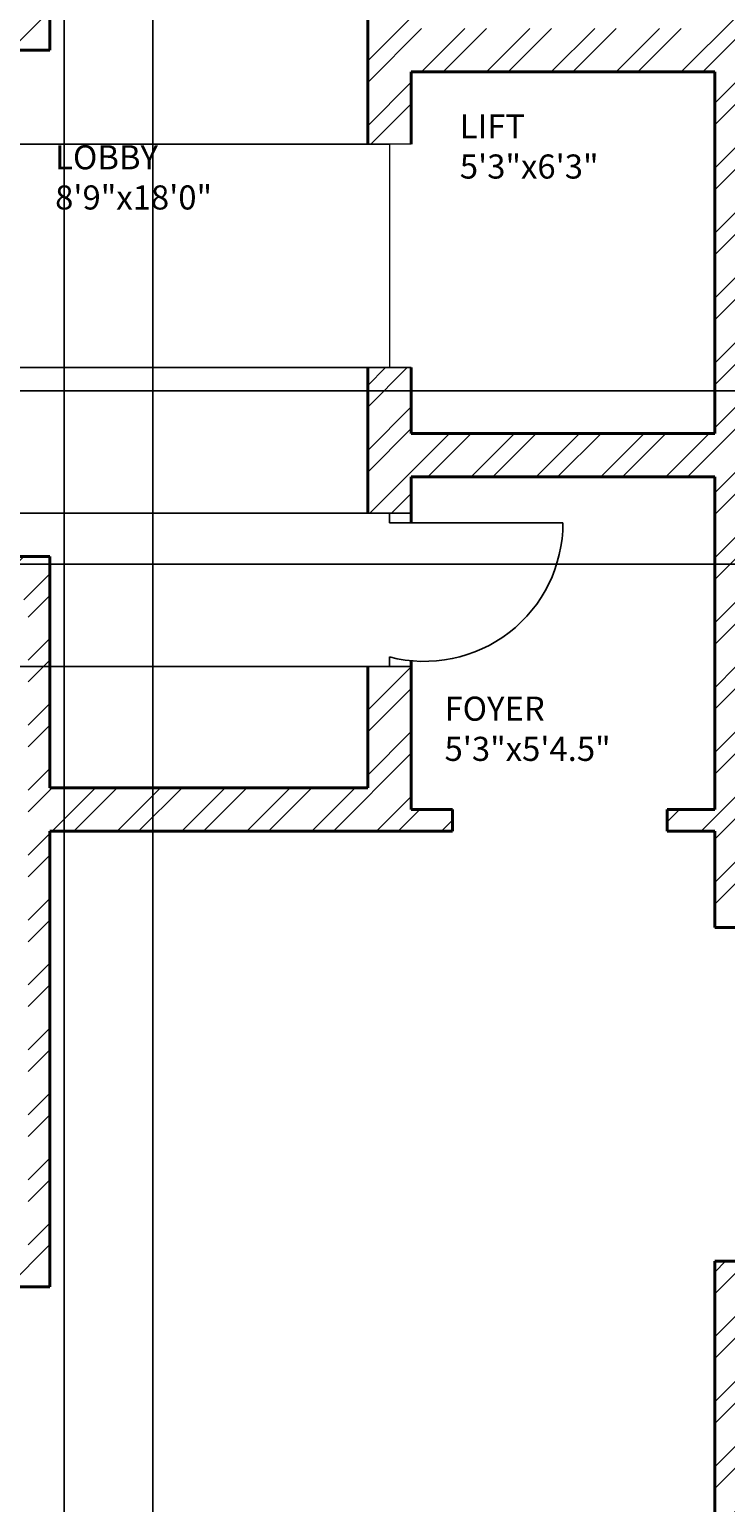
# Model space of a CAD drawing. Units: inches. Extents: x 1601 to 2297, y 1496 to 2631.
# Tile 15 of 57: x 1889 to 2033, y 1835 to 2141. Entities that reach past the tile are written whole.
import ezdxf

# ---------------------------------------------------------------- set-up
doc = ezdxf.new("R2010")
doc.units = ezdxf.units.IN
for name, color, linetype, lineweight in [('A-ANNO-DIMS', 2, 'Continuous', 18), ('A-AREA-IDEN', 7, 'Continuous', 18), ('A-DOOR', 21, 'Continuous', 25), ('A-FLOR-EVTR', 4, 'Continuous', 20), ('A-WALL', 7, 'Continuous', 40), ('A-WALL-PATT', 215, 'Continuous', 13)]:
    doc.layers.add(name, color=color, linetype=linetype, lineweight=lineweight)
doc.styles.get("Standard").update_dxf_attribs({"font": 'arial.ttf'})
doc.dimstyles.get("Standard").update_dxf_attribs({"dimtxt": 0.18, "dimasz": 0.18, "dimexe": 0.18, "dimexo": 0.0625, "dimgap": 0.09, "dimtad": 0, "dimtih": 1, "dimtoh": 1, "dimdec": 4, "dimzin": 0, "dimdsep": 46, "dimtxsty": 'Standard', "dimcen": 0.09, "dimadec": 0, "dimazin": 0, "dimtfac": 1, "dimtdec": 4, "dimtofl": 0, "dimtmove": 0, "dimatfit": 3, "dimfxl": 1, "dimtolj": 1, "dimtzin": 0, "dimarcsym": 0})

# ---------------------------------------------------------------- blocks, each defined once
blk = doc.blocks.new('*D42')
at = {"layer": 'A-ANNO-DIMS', "color": 0, "lineweight": -2, "transparency": 16777216}
for p, q in [((2177.97, 2065.7), (1637.31, 2065.7)), ((1637.49, 2065.52), (1637.49, 2047.88)), ((1637.49, 2029.88), (1637.49, 2047.51)), ((2177.97, 2029.7), (1637.31, 2029.7))]:
    blk.add_line(p, q, dxfattribs=at)
at = {"layer": 'A-ANNO-DIMS', "color": 0, "transparency": 16777216}
for points in [[(1637.46, 2065.52), (1637.52, 2065.52), (1637.49, 2065.7)], [(1637.46, 2029.88), (1637.52, 2029.88), (1637.49, 2029.7)]]:
    blk.add_solid(points, dxfattribs=at)
at = {"layer": 'Defpoints', "color": 0, "transparency": 16777216}
for p in [(1637.49, 2065.7), (2178.04, 2065.7), (2178.04, 2029.7)]:
    blk.add_point(p, dxfattribs=at)
at = {"layer": 'A-ANNO-DIMS', "color": 0, "transparency": 16777216, "insert": (1637.49, 2047.7), "char_height": 0.18, "attachment_point": 5}
blk.add_mtext('\\A1;36', dxfattribs=at)
blk = doc.blocks.new('*D44')
at = {"layer": 'A-ANNO-DIMS', "color": 0, "lineweight": -2, "transparency": 16777216}
for p, q in [((1958.97, 2116.84), (1637.31, 2116.84)), ((1637.49, 2116.66), (1637.49, 2093.85)), ((1637.49, 2070.67), (1637.49, 2093.48)), ((1958.97, 2070.49), (1637.31, 2070.49))]:
    blk.add_line(p, q, dxfattribs=at)
at = {"layer": 'A-ANNO-DIMS', "color": 0, "transparency": 16777216}
for points in [[(1637.46, 2116.66), (1637.52, 2116.66), (1637.49, 2116.84)], [(1637.46, 2070.67), (1637.52, 2070.67), (1637.49, 2070.49)]]:
    blk.add_solid(points, dxfattribs=at)
at = {"layer": 'Defpoints', "color": 0, "transparency": 16777216}
for p in [(1637.49, 2116.84), (1959.04, 2116.84), (1959.04, 2070.49)]:
    blk.add_point(p, dxfattribs=at)
at = {"layer": 'A-ANNO-DIMS', "color": 0, "transparency": 16777216, "insert": (1637.49, 2093.67), "char_height": 0.18, "attachment_point": 5}
blk.add_mtext('\\A1;46.34', dxfattribs=at)
blk = doc.blocks.new('*D45')
at = {"layer": 'A-ANNO-DIMS', "color": 0, "lineweight": -2, "transparency": 16777216}
for p, q in [((1958.97, 2040.3), (1637.31, 2040.3)), ((1637.49, 2040.12), (1637.49, 2024.57)), ((1637.49, 2008.66), (1637.49, 2024.21)), ((1958.97, 2008.48), (1637.31, 2008.48))]:
    blk.add_line(p, q, dxfattribs=at)
at = {"layer": 'A-ANNO-DIMS', "color": 0, "transparency": 16777216}
for points in [[(1637.46, 2040.12), (1637.52, 2040.12), (1637.49, 2040.3)], [(1637.46, 2008.66), (1637.52, 2008.66), (1637.49, 2008.48)]]:
    blk.add_solid(points, dxfattribs=at)
at = {"layer": 'Defpoints', "color": 0, "transparency": 16777216}
for p in [(1637.49, 2040.3), (1959.04, 2040.3), (1959.04, 2008.48)]:
    blk.add_point(p, dxfattribs=at)
at = {"layer": 'A-ANNO-DIMS', "color": 0, "transparency": 16777216, "insert": (1637.49, 2024.39), "char_height": 0.18, "attachment_point": 5}
blk.add_mtext('\\A1;31.83', dxfattribs=at)
blk = doc.blocks.new('*D50')
at = {"layer": 'A-ANNO-DIMS', "color": 0, "lineweight": -2, "transparency": 16777216}
for p, q in [((1895.99, 2374.33), (1895.99, 1513.75)), ((1914.39, 2374.33), (1914.39, 1513.75)), ((1896.17, 1513.93), (1904.87, 1513.93)), ((1914.21, 1513.93), (1905.5, 1513.93))]:
    blk.add_line(p, q, dxfattribs=at)
at = {"layer": 'A-ANNO-DIMS', "color": 0, "transparency": 16777216}
for points in [[(1896.17, 1513.96), (1896.17, 1513.9), (1895.99, 1513.93)], [(1914.21, 1513.96), (1914.21, 1513.9), (1914.39, 1513.93)]]:
    blk.add_solid(points, dxfattribs=at)
at = {"layer": 'Defpoints', "color": 0, "transparency": 16777216}
for p in [(1895.99, 2374.4), (1914.39, 2374.4), (1914.39, 1513.93)]:
    blk.add_point(p, dxfattribs=at)
at = {"layer": 'A-ANNO-DIMS', "color": 0, "transparency": 16777216, "insert": (1905.19, 1513.93), "char_height": 0.18, "attachment_point": 5}
blk.add_mtext('\\A1;18.4', dxfattribs=at)

msp = doc.modelspace()

# ---------------------------------------------------------------- hatches: boundary and pattern name
at = {"layer": 'A-WALL-PATT'}
h = msp.add_hatch(dxfattribs=at)
h.set_pattern_fill('ANSI32', color=256)
h.paths.add_polyline_path([(1842.0336, 2528.0767), (1842.0336, 2532.3254), (1686.0373, 2532.3254), (1686.0373, 2492.9493), (1695.0373, 2492.9493), (1695.0373, 2523.3254), (1827.0373, 2523.3254), (1827.0373, 2416.8254), (1834.6225, 2416.8254), (1834.6225, 2419.0754), (1834.6225, 2421.3254), (1831.5373, 2421.3254), (1831.5373, 2523.3254), (1842.0336, 2523.3254)])
h.paths.add_polyline_path([(1695.0373, 2432.9493), (1686.0373, 2432.9493), (1686.0373, 2325.989), (1695.0373, 2325.989), (1695.0373, 2347.8254), (1827.0373, 2347.8254), (1827.0373, 2287.8254), (1823.2991, 2287.8254), (1823.2991, 2283.3254), (1847.9422, 2283.3254), (1847.9422, 2285.5754), (1847.9422, 2287.8254), (1831.5373, 2287.8254), (1831.5373, 2347.8254), (1846.9946, 2347.8254), (1846.9946, 2350.0754), (1846.9946, 2352.3254), (1695.0373, 2352.3254)])
h.paths.add_polyline_path([(1807.1169, 1573.5395), (2055.0405, 1573.5395), (2055.0405, 1610.6322), (1807.1169, 1610.6322)], flags=9)
h.paths.add_polyline_path([(1841.1631, 1712.7967), (1870.3957, 1712.7967), (1870.3957, 1731.454), (1841.1631, 1731.454)], flags=9)
h.paths.add_polyline_path([(2144.3862, 1772.185), (2191.0233, 1772.185), (2191.0233, 1790.8423), (2144.3862, 1790.8423)], flags=9)
h.paths.add_polyline_path([(2143.0128, 1827.3312), (2177.9958, 1827.3312), (2177.9958, 1845.9886), (2143.0128, 1845.9886)], flags=9)
h.paths.add_polyline_path([(2041.2439, 1833.5691), (2070.8516, 1833.5691), (2070.8516, 1852.2264), (2041.2439, 1852.2264)], flags=9)
h.paths.add_polyline_path([(2097.2791, 1947.0598), (2134.2061, 1947.0598), (2134.2061, 1965.7171), (2097.2791, 1965.7171)], flags=9)
h.paths.add_polyline_path([(2214.995, 1904.3124), (2214.995, 1942.2899), (2196.3376, 1942.2899), (2196.3376, 1904.3124)], flags=9)
h.paths.add_polyline_path([(2186.6284, 2043.8031), (2219.7935, 2043.8031), (2219.7935, 2062.4605), (2186.6284, 2062.4605)], flags=9)
h.paths.add_polyline_path([(2064.0877, 2031.616), (2097.4949, 2031.616), (2097.4949, 2050.2734), (2064.0877, 2050.2734)], flags=9)
h.paths.add_polyline_path([(1973.1349, 1986.0688), (2008.4009, 1986.0688), (2008.4009, 2004.7261), (1973.1349, 2004.7261)], flags=9)
h.paths.add_polyline_path([(1976.3676, 2106.9635), (2005.7469, 2106.9635), (2005.7469, 2125.6209), (1976.3676, 2125.6209)], flags=9)
h.paths.add_polyline_path([(1991.7852, 2180.4863), (2027.0513, 2180.4863), (2027.0513, 2199.1437), (1991.7852, 2199.1437)], flags=9)
h.paths.add_polyline_path([(2106.1801, 2187.9359), (2152.2101, 2187.9359), (2152.2101, 2206.5932), (2106.1801, 2206.5932)], flags=9)
h.paths.add_polyline_path([(2148.6686, 2262.2542), (2182.318, 2262.2542), (2182.318, 2280.9115), (2148.6686, 2280.9115)], flags=9)
h.paths.add_polyline_path([(2041.6327, 2252.8147), (2071.2405, 2252.8147), (2071.2405, 2271.4721), (2041.6327, 2271.4721)], flags=9)
h.paths.add_polyline_path([(2063.9734, 2375.4265), (2100.9004, 2375.4265), (2100.9004, 2394.0839), (2063.9734, 2394.0839)], flags=9)
h.paths.add_polyline_path([(2216.4955, 2330.9748), (2216.4955, 2370.2654), (2197.8381, 2370.2654), (2197.8381, 2330.9748)], flags=9)
h.paths.add_polyline_path([(2179.1416, 2485.8687), (2212.3067, 2485.8687), (2212.3067, 2504.5261), (2179.1416, 2504.5261)], flags=9)
h.paths.add_polyline_path([(2078.7442, 2471.1516), (2112.1514, 2471.1516), (2112.1514, 2489.809), (2078.7442, 2489.809)], flags=9)
h.paths.add_polyline_path([(1915.9631, 2329.4668), (1952.8902, 2329.4668), (1952.8902, 2348.1241), (1915.9631, 2348.1241)], flags=9)
h.paths.add_polyline_path([(1904.3189, 2499.6709), (1940.4512, 2499.6709), (1940.4512, 2518.3282), (1904.3189, 2518.3282)], flags=9)
h.paths.add_polyline_path([(1892.3665, 2100.4595), (1925.6374, 2100.4595), (1925.6374, 2119.1169), (1892.3665, 2119.1169)], flags=9)
h.paths.add_polyline_path([(1909.2984, 1805.9631), (1946.2254, 1805.9631), (1946.2254, 1824.6205), (1909.2984, 1824.6205)], flags=9)
h.paths.add_polyline_path([(1934.6056, 1658.616), (1970.738, 1658.616), (1970.738, 1677.2733), (1934.6056, 1677.2733)], flags=9)
h.paths.add_polyline_path([(1711.2052, 1789.8902), (1750.0456, 1789.8902), (1750.0456, 1808.5476), (1711.2052, 1808.5476)], flags=9)
h.paths.add_polyline_path([(1742.7874, 1854.6743), (1771.9449, 1854.6743), (1771.9449, 1873.3317), (1742.7874, 1873.3317)], flags=9)
h.paths.add_polyline_path([(1807.3592, 1997.7912), (1850.1116, 1997.7912), (1850.1116, 2016.4486), (1807.3592, 2016.4486)], flags=9)
h.paths.add_polyline_path([(1717.4579, 2237.7844), (1760.2103, 2237.7844), (1760.2103, 2256.4417), (1717.4579, 2256.4417)], flags=9)
h.paths.add_polyline_path([(1780.9285, 2324.0623), (1810.086, 2324.0623), (1810.086, 2342.7197), (1780.9285, 2342.7197)], flags=25)
h.paths.add_polyline_path([(1837.696, 2449.2024), (1866.9286, 2449.2024), (1866.9286, 2467.8598), (1837.696, 2467.8598)], flags=9)
h.paths.add_polyline_path([(1712.7752, 2484.9404), (1751.6156, 2484.9404), (1751.6156, 2503.5977), (1712.7752, 2503.5977)], flags=25)
h = msp.add_hatch(dxfattribs=at)
h.set_pattern_fill('ANSI32', color=256)
h.paths.add_polyline_path([(1973.9371, 2211.3254), (1893.0373, 2211.3254), (1893.0373, 2287.8254), (1884.6167, 2287.8254), (1884.6167, 2285.5754), (1884.6167, 2283.3254), (1888.5373, 2283.3254), (1888.5373, 2145.3254), (1695.0373, 2145.3254), (1695.0373, 2173.8724), (1690.5373, 2173.8724), (1686.0373, 2173.8724), (1686.0373, 2136.3254), (1722.5687, 2136.3254), (1722.5687, 2117.4352), (1731.5687, 2117.4352), (1731.5687, 2136.3254), (1893.0373, 2136.3254), (1893.0373, 2202.3254), (1959.0373, 2202.3254), (1959.0373, 2182.1303), (1968.0373, 2182.1303), (1968.0373, 2202.3254), (1973.9371, 2202.3254)])
h.paths.add_polyline_path([(2094.0373, 2274.6364), (2096.4294, 2274.6364), (2096.4294, 2276.8864), (2096.4294, 2279.1364), (2094.0373, 2279.1364), (2094.0373, 2290.8254), (2094.0373, 2295.3254), (2089.5373, 2295.3254), (2089.5373, 2230.8254), (2035.5373, 2230.8254), (2035.5373, 2299.8254), (2031.0373, 2299.8254), (2031.0373, 2211.3254), (2023.0065, 2211.3254), (2023.0065, 2202.3254), (2031.0373, 2202.3254), (2031.0373, 2140.8254), (1968.0373, 2140.8254), (1968.0373, 2145.9106), (1963.5373, 2145.9106), (1959.0373, 2145.9106), (1959.0373, 2116.839), (1963.5373, 2116.839), (1968.0373, 2116.839), (1968.0373, 2131.8254), (2031.0373, 2131.8254), (2031.0373, 2094.3254), (2031.0373, 2085.3254), (2031.0373, 2056.8254), (1968.0373, 2056.8254), (1968.0373, 2070.4947), (1963.5373, 2070.4947), (1959.0373, 2070.4947), (1959.0373, 2040.3029), (1968.0373, 2040.3029), (1968.0373, 2047.8254), (2031.0373, 2047.8254), (2031.0373, 1983.3254), (2031.0373, 1978.8254), (2021.1979, 1978.8254), (2021.1979, 1974.3254), (2031.0373, 1974.3254), (2031.0373, 1954.3528), (2035.5373, 1954.3528), (2035.5373, 1974.3254), (2035.5373, 1981.8254), (2055.5513, 1981.8254), (2055.5513, 1986.3254), (2035.5373, 1986.3254), (2035.5373, 2047.8254), (2040.0373, 2047.8254), (2040.0373, 2085.3254), (2040.0373, 2094.3254), (2040.0373, 2140.8254), (2035.5373, 2140.8254), (2035.5373, 2226.3254), (2089.5373, 2226.3254), (2094.0373, 2226.3254)])
h.paths.add_polyline_path([(2226.0373, 2230.8254), (2134.5373, 2230.8254), (2134.5373, 2233.5437), (2130.0373, 2233.5437), (2130.0373, 2226.3254), (2134.5373, 2226.3254), (2226.0373, 2226.3254)])
h.paths.add_polyline_path([(1807.1169, 1573.5395), (2055.0405, 1573.5395), (2055.0405, 1610.6322), (1807.1169, 1610.6322)], flags=9)
h.paths.add_polyline_path([(1841.1631, 1712.7967), (1870.3957, 1712.7967), (1870.3957, 1731.454), (1841.1631, 1731.454)], flags=9)
h.paths.add_polyline_path([(2144.3862, 1772.185), (2191.0233, 1772.185), (2191.0233, 1790.8423), (2144.3862, 1790.8423)], flags=9)
h.paths.add_polyline_path([(2143.0128, 1827.3312), (2177.9958, 1827.3312), (2177.9958, 1845.9886), (2143.0128, 1845.9886)], flags=9)
h.paths.add_polyline_path([(2041.2439, 1833.5691), (2070.8516, 1833.5691), (2070.8516, 1852.2264), (2041.2439, 1852.2264)], flags=9)
h.paths.add_polyline_path([(2097.2791, 1947.0598), (2134.2061, 1947.0598), (2134.2061, 1965.7171), (2097.2791, 1965.7171)], flags=9)
h.paths.add_polyline_path([(2214.995, 1904.3124), (2214.995, 1942.2899), (2196.3376, 1942.2899), (2196.3376, 1904.3124)], flags=9)
h.paths.add_polyline_path([(2186.6284, 2043.8031), (2219.7935, 2043.8031), (2219.7935, 2062.4605), (2186.6284, 2062.4605)], flags=9)
h.paths.add_polyline_path([(2064.0877, 2031.616), (2097.4949, 2031.616), (2097.4949, 2050.2734), (2064.0877, 2050.2734)], flags=9)
h.paths.add_polyline_path([(1973.1349, 1986.0688), (2008.4009, 1986.0688), (2008.4009, 2004.7261), (1973.1349, 2004.7261)], flags=25)
h.paths.add_polyline_path([(1976.3676, 2106.9635), (2005.7469, 2106.9635), (2005.7469, 2125.6209), (1976.3676, 2125.6209)], flags=25)
h.paths.add_polyline_path([(1991.7852, 2180.4863), (2027.0513, 2180.4863), (2027.0513, 2199.1437), (1991.7852, 2199.1437)], flags=25)
h.paths.add_polyline_path([(2106.1801, 2187.9359), (2152.2101, 2187.9359), (2152.2101, 2206.5932), (2106.1801, 2206.5932)], flags=9)
h.paths.add_polyline_path([(2148.6686, 2262.2542), (2182.318, 2262.2542), (2182.318, 2280.9115), (2148.6686, 2280.9115)], flags=9)
h.paths.add_polyline_path([(2041.6327, 2252.8147), (2071.2405, 2252.8147), (2071.2405, 2271.4721), (2041.6327, 2271.4721)], flags=25)
h.paths.add_polyline_path([(2063.9734, 2375.4265), (2100.9004, 2375.4265), (2100.9004, 2394.0839), (2063.9734, 2394.0839)], flags=9)
h.paths.add_polyline_path([(2216.4955, 2330.9748), (2216.4955, 2370.2654), (2197.8381, 2370.2654), (2197.8381, 2330.9748)], flags=9)
h.paths.add_polyline_path([(2179.1416, 2485.8687), (2212.3067, 2485.8687), (2212.3067, 2504.5261), (2179.1416, 2504.5261)], flags=9)
h.paths.add_polyline_path([(2078.7442, 2471.1516), (2112.1514, 2471.1516), (2112.1514, 2489.809), (2078.7442, 2489.809)], flags=9)
h.paths.add_polyline_path([(1915.9631, 2329.4668), (1952.8902, 2329.4668), (1952.8902, 2348.1241), (1915.9631, 2348.1241)], flags=9)
h.paths.add_polyline_path([(1904.3189, 2499.6709), (1940.4512, 2499.6709), (1940.4512, 2518.3282), (1904.3189, 2518.3282)], flags=9)
h.paths.add_polyline_path([(1892.3665, 2100.4595), (1925.6374, 2100.4595), (1925.6374, 2119.1169), (1892.3665, 2119.1169)], flags=9)
h.paths.add_polyline_path([(1909.2984, 1805.9631), (1946.2254, 1805.9631), (1946.2254, 1824.6205), (1909.2984, 1824.6205)], flags=9)
h.paths.add_polyline_path([(1934.6056, 1658.616), (1970.738, 1658.616), (1970.738, 1677.2733), (1934.6056, 1677.2733)], flags=9)
h.paths.add_polyline_path([(1711.2052, 1789.8902), (1750.0456, 1789.8902), (1750.0456, 1808.5476), (1711.2052, 1808.5476)], flags=9)
h.paths.add_polyline_path([(1742.7874, 1854.6743), (1771.9449, 1854.6743), (1771.9449, 1873.3317), (1742.7874, 1873.3317)], flags=9)
h.paths.add_polyline_path([(1807.3592, 1997.7912), (1850.1116, 1997.7912), (1850.1116, 2016.4486), (1807.3592, 2016.4486)], flags=9)
h.paths.add_polyline_path([(1717.4579, 2237.7844), (1760.2103, 2237.7844), (1760.2103, 2256.4417), (1717.4579, 2256.4417)], flags=25)
h.paths.add_polyline_path([(1780.9285, 2324.0623), (1810.086, 2324.0623), (1810.086, 2342.7197), (1780.9285, 2342.7197)], flags=9)
h.paths.add_polyline_path([(1837.696, 2449.2024), (1866.9286, 2449.2024), (1866.9286, 2467.8598), (1837.696, 2467.8598)], flags=9)
h.paths.add_polyline_path([(1712.7752, 2484.9404), (1751.6156, 2484.9404), (1751.6156, 2503.5977), (1712.7752, 2503.5977)], flags=9)
h = msp.add_hatch(dxfattribs=at)
h.set_pattern_fill('ANSI32', color=256)
h.paths.add_polyline_path([(2230.5373, 1861.8254), (2182.5373, 1861.8254), (2182.5373, 1885.3637), (2178.0373, 1885.3637), (2178.0373, 1861.8254), (2166.0373, 1861.8254), (2134.5373, 1861.8254), (2130.0373, 1861.8254), (2130.0373, 1841.4682), (2126.8833, 1841.4682), (2126.8833, 1836.9682), (2130.0373, 1836.9682), (2130.0373, 1822.7302), (2134.5373, 1822.7302), (2134.5373, 1857.3254), (2166.0373, 1857.3254), (2226.0373, 1857.3254), (2226.0373, 1846.1155), (2230.5373, 1846.1155)])
h.paths.add_polyline_path([(2226.0373, 1797.3254), (2134.5373, 1797.3254), (2134.5373, 1800.6636), (2132.2873, 1800.6636), (2130.0373, 1800.6636), (2130.0373, 1797.3254), (2130.0373, 1792.8254), (2167.7264, 1792.8254), (2226.0373, 1792.8254)])
h.paths.add_polyline_path([(2230.5373, 1822.1155), (2226.0373, 1822.1155), (2226.0373, 1760.8563), (2230.5373, 1760.8563)])
h.paths.add_polyline_path([(2230.5373, 1700.8563), (2226.0373, 1700.8563), (2226.0373, 1644.3254), (2140.2517, 1644.3254), (2140.2517, 1635.3254), (2230.5373, 1635.3254)])
h.paths.add_polyline_path([(2080.2517, 1639.8254), (2080.2517, 1644.3254), (2035.5373, 1644.3254), (2035.5373, 1792.8254), (2094.0373, 1792.8254), (2094.0373, 1797.3254), (2094.0373, 1836.9682), (2097.1057, 1836.9682), (2097.1057, 1839.2182), (2097.1057, 1841.4682), (2094.0373, 1841.4682), (2094.0373, 1862.2276), (2089.5373, 1862.2276), (2089.5373, 1797.3254), (2035.5373, 1797.3254), (2035.5373, 1857.3254), (2035.5373, 1885.0916), (2031.0373, 1885.0916), (2031.0373, 1710.3254), (2012.329, 1710.3254), (2012.329, 1701.3254), (2031.0373, 1701.3254), (2031.0373, 1644.3254), (2031.0373, 1635.3254), (2080.2517, 1635.3254)])
h.paths.add_polyline_path([(1836.0373, 1653.2033), (1842.6171, 1653.2033), (1842.6171, 1657.7033), (1842.6171, 1662.2033), (1831.5373, 1662.2033), (1831.5373, 1764.2033), (1835.3881, 1764.2033), (1835.3881, 1766.4533), (1835.3881, 1768.7033), (1831.5373, 1768.7033), (1827.0373, 1768.7033), (1827.0373, 1662.2033), (1827.0373, 1635.3254), (1836.0373, 1635.3254)])
h.paths.add_polyline_path([(1893.0373, 1701.3254), (1907.193, 1701.3254), (1907.193, 1705.8254), (1907.193, 1710.3254), (1893.0373, 1710.3254), (1893.0373, 1819.8254), (1882.6444, 1819.8254), (1882.6444, 1817.5754), (1882.6444, 1815.3254), (1888.5373, 1815.3254), (1888.5373, 1662.2033), (1884.0373, 1662.2033), (1866.6171, 1662.2033), (1866.6171, 1653.2033), (1882.391, 1653.2033), (1884.0373, 1653.2033), (1884.0373, 1635.3254), (1893.0373, 1635.3254)])
h.paths.add_polyline_path([(1739.3335, 1639.8254), (1739.3335, 1644.3254), (1695.0373, 1644.3254), (1695.0373, 1702.0135), (1690.5373, 1702.0135), (1686.0373, 1702.0135), (1686.0373, 1635.3254), (1739.3335, 1635.3254)])
h.paths.add_polyline_path([(1827.0373, 1644.3254), (1799.3335, 1644.3254), (1799.3335, 1635.3254), (1827.0373, 1635.3254)])
h.paths.add_polyline_path([(1695.0373, 1815.3254), (1849.2759, 1815.3254), (1849.2759, 1819.8254), (1807.5373, 1819.8254), (1807.5373, 1879.8254), (1851.1533, 1879.8254), (1851.1533, 1882.0754), (1851.1533, 1884.3254), (1799.3405, 1884.3254), (1799.3405, 1882.0754), (1799.3405, 1879.8254), (1803.0373, 1879.8254), (1803.0373, 1819.8254), (1695.0373, 1819.8254), (1695.0373, 1835.0458), (1690.5373, 1835.0458), (1686.0373, 1835.0458), (1686.0373, 1766.1753), (1695.0373, 1766.1753)])
h.paths.add_polyline_path([(1775.8157, 1884.3254), (1695.0373, 1884.3254), (1695.0373, 1912.9526), (1690.5373, 1912.9526), (1686.0373, 1912.9526), (1686.0373, 1859.0458), (1695.0373, 1859.0458), (1695.0373, 1879.8254), (1775.8157, 1879.8254)])
h.paths.add_polyline_path([(1893.0373, 2031.3254), (1731.5687, 2031.3254), (1731.5687, 2057.4352), (1722.5687, 2057.4352), (1722.5687, 2031.3254), (1686.0373, 2031.3254), (1686.0373, 1972.9526), (1695.0373, 1972.9526), (1695.0373, 2022.3254), (1888.5373, 2022.3254), (1888.5373, 1884.3254), (1883.4996, 1884.3254), (1883.4996, 1879.8254), (1893.0373, 1879.8254), (1893.0373, 1974.3254), (1976.6199, 1974.3254), (1976.6199, 1978.8254), (1968.0373, 1978.8254), (1968.0373, 1983.3254), (1968.0373, 2008.4756), (1963.5373, 2008.4756), (1959.0373, 2008.4756), (1959.0373, 1983.3254), (1893.0373, 1983.3254)])
h.paths.add_polyline_path([(2230.5373, 2140.4745), (2226.0373, 2140.4745), (2226.0373, 2094.3254), (2040.0373, 2094.3254), (2040.0373, 2085.3254), (2178.0373, 2085.3254), (2178.0373, 2065.6965), (2182.5373, 2065.6965), (2182.5373, 2085.3254), (2226.0373, 2085.3254), (2226.0373, 1986.3254), (2211.2679, 1986.3254), (2211.2679, 1981.8254), (2230.5373, 1981.8254)])
h.paths.add_polyline_path([(2187.6292, 1986.3254), (2182.5373, 1986.3254), (2182.5373, 2029.6965), (2178.0373, 2029.6965), (2178.0373, 1986.3254), (2099.05, 1986.3254), (2099.05, 1981.8254), (2178.0373, 1981.8254), (2178.0373, 1969.3637), (2182.5373, 1969.3637), (2182.5373, 1981.8254), (2187.6292, 1981.8254), (2187.6292, 1984.0754)])
h.paths.add_polyline_path([(1807.1169, 1573.5395), (2055.0405, 1573.5395), (2055.0405, 1610.6322), (1807.1169, 1610.6322)], flags=9)
h.paths.add_polyline_path([(1841.1631, 1712.7967), (1870.3957, 1712.7967), (1870.3957, 1731.454), (1841.1631, 1731.454)], flags=9)
h.paths.add_polyline_path([(2144.3862, 1772.185), (2191.0233, 1772.185), (2191.0233, 1790.8423), (2144.3862, 1790.8423)], flags=9)
h.paths.add_polyline_path([(2143.0128, 1827.3312), (2177.9958, 1827.3312), (2177.9958, 1845.9886), (2143.0128, 1845.9886)], flags=25)
h.paths.add_polyline_path([(2041.2439, 1833.5691), (2070.8516, 1833.5691), (2070.8516, 1852.2264), (2041.2439, 1852.2264)], flags=25)
h.paths.add_polyline_path([(2097.2791, 1947.0598), (2134.2061, 1947.0598), (2134.2061, 1965.7171), (2097.2791, 1965.7171)], flags=9)
h.paths.add_polyline_path([(2214.995, 1904.3124), (2214.995, 1942.2899), (2196.3376, 1942.2899), (2196.3376, 1904.3124)], flags=9)
h.paths.add_polyline_path([(2186.6284, 2043.8031), (2219.7935, 2043.8031), (2219.7935, 2062.4605), (2186.6284, 2062.4605)], flags=25)
h.paths.add_polyline_path([(2064.0877, 2031.616), (2097.4949, 2031.616), (2097.4949, 2050.2734), (2064.0877, 2050.2734)], flags=25)
h.paths.add_polyline_path([(1973.1349, 1986.0688), (2008.4009, 1986.0688), (2008.4009, 2004.7261), (1973.1349, 2004.7261)], flags=9)
h.paths.add_polyline_path([(1976.3676, 2106.9635), (2005.7469, 2106.9635), (2005.7469, 2125.6209), (1976.3676, 2125.6209)], flags=9)
h.paths.add_polyline_path([(1991.7852, 2180.4863), (2027.0513, 2180.4863), (2027.0513, 2199.1437), (1991.7852, 2199.1437)], flags=9)
h.paths.add_polyline_path([(2106.1801, 2187.9359), (2152.2101, 2187.9359), (2152.2101, 2206.5932), (2106.1801, 2206.5932)], flags=9)
h.paths.add_polyline_path([(2148.6686, 2262.2542), (2182.318, 2262.2542), (2182.318, 2280.9115), (2148.6686, 2280.9115)], flags=9)
h.paths.add_polyline_path([(2041.6327, 2252.8147), (2071.2405, 2252.8147), (2071.2405, 2271.4721), (2041.6327, 2271.4721)], flags=9)
h.paths.add_polyline_path([(2063.9734, 2375.4265), (2100.9004, 2375.4265), (2100.9004, 2394.0839), (2063.9734, 2394.0839)], flags=9)
h.paths.add_polyline_path([(2216.4955, 2330.9748), (2216.4955, 2370.2654), (2197.8381, 2370.2654), (2197.8381, 2330.9748)], flags=9)
h.paths.add_polyline_path([(2179.1416, 2485.8687), (2212.3067, 2485.8687), (2212.3067, 2504.5261), (2179.1416, 2504.5261)], flags=9)
h.paths.add_polyline_path([(2078.7442, 2471.1516), (2112.1514, 2471.1516), (2112.1514, 2489.809), (2078.7442, 2489.809)], flags=9)
h.paths.add_polyline_path([(1915.9631, 2329.4668), (1952.8902, 2329.4668), (1952.8902, 2348.1241), (1915.9631, 2348.1241)], flags=9)
h.paths.add_polyline_path([(1904.3189, 2499.6709), (1940.4512, 2499.6709), (1940.4512, 2518.3282), (1904.3189, 2518.3282)], flags=9)
h.paths.add_polyline_path([(1892.3665, 2100.4595), (1925.6374, 2100.4595), (1925.6374, 2119.1169), (1892.3665, 2119.1169)], flags=9)
h.paths.add_polyline_path([(1909.2984, 1805.9631), (1946.2254, 1805.9631), (1946.2254, 1824.6205), (1909.2984, 1824.6205)], flags=9)
h.paths.add_polyline_path([(1934.6056, 1658.616), (1970.738, 1658.616), (1970.738, 1677.2733), (1934.6056, 1677.2733)], flags=9)
h.paths.add_polyline_path([(1711.2052, 1789.8902), (1750.0456, 1789.8902), (1750.0456, 1808.5476), (1711.2052, 1808.5476)], flags=25)
h.paths.add_polyline_path([(1742.7874, 1854.6743), (1771.9449, 1854.6743), (1771.9449, 1873.3317), (1742.7874, 1873.3317)], flags=25)
h.paths.add_polyline_path([(1807.3592, 1997.7912), (1850.1116, 1997.7912), (1850.1116, 2016.4486), (1807.3592, 2016.4486)], flags=25)
h.paths.add_polyline_path([(1717.4579, 2237.7844), (1760.2103, 2237.7844), (1760.2103, 2256.4417), (1717.4579, 2256.4417)], flags=9)
h.paths.add_polyline_path([(1780.9285, 2324.0623), (1810.086, 2324.0623), (1810.086, 2342.7197), (1780.9285, 2342.7197)], flags=9)
h.paths.add_polyline_path([(1837.696, 2449.2024), (1866.9286, 2449.2024), (1866.9286, 2467.8598), (1837.696, 2467.8598)], flags=9)
h.paths.add_polyline_path([(1712.7752, 2484.9404), (1751.6156, 2484.9404), (1751.6156, 2503.5977), (1712.7752, 2503.5977)], flags=9)

# ---------------------------------------------------------------- linework, layer by layer
at = {"layer": 'A-DOOR'}
for p, q in [((1959.0373, 2040.3029), (1968.0373, 2040.3029)), ((1968.0373, 2040.3029), (1963.5373, 2040.3029)), ((1963.5373, 2040.3029), (1963.5373, 2038.3029)), ((1968.0373, 2040.3029), (1968.0373, 2040.3029)), ((1963.5373, 2038.3029), (1999.5373, 2038.3029)), ((1959.0373, 2008.4756), (1968.0373, 2008.4756)), ((1963.5373, 2008.4756), (1963.5373, 2010.4756)), ((1968.0373, 2008.4756), (1963.5373, 2008.4756))]:
    msp.add_line(p, q, dxfattribs=at)
msp.add_arc((1970.7823, 2038.3029), 28.755, 255.406703, 0, dxfattribs=at)
at = {"layer": 'A-FLOR-EVTR'}
for p, q in [((1968.0373, 2116.839), (1959.0373, 2116.839)), ((1959.0373, 2116.839), (1963.5373, 2116.839)), ((1963.5373, 2116.839), (1963.5373, 2070.4947)), ((1963.5373, 2070.4947), (1959.0373, 2070.4947)), ((1959.0373, 2070.4947), (1968.0373, 2070.4947)), ((1968.0373, 2070.4947), (1963.5373, 2070.4947))]:
    msp.add_line(p, q, dxfattribs=at)
at = {"layer": 'A-WALL'}
for p, q in [((1893.0373, 2202.3254), (1893.0373, 2136.3254)), ((1959.0373, 2145.9106), (1959.0373, 2116.839)), ((1731.5687, 2136.3254), (1893.0373, 2136.3254)), ((1968.0373, 2131.8254), (2031.0373, 2131.8254)), ((1968.0373, 2116.839), (1968.0373, 2131.8254)), ((2031.0373, 2131.8254), (2031.0373, 2094.3254)), ((2031.0373, 2094.3254), (2031.0373, 2085.3254)), ((2031.0373, 2085.3254), (2031.0373, 2056.8254)), ((1959.0373, 2070.4947), (1959.0373, 2040.3029)), ((1968.0373, 2056.8254), (1968.0373, 2070.4947)), ((1968.0373, 2056.8254), (2031.0373, 2056.8254)), ((1968.0373, 2047.8254), (2031.0373, 2047.8254)), ((2031.0373, 2047.8254), (1968.0373, 2047.8254)), ((1968.0373, 2038.3029), (1968.0373, 2047.8254)), ((2031.0373, 2047.8254), (2031.0373, 2047.8254)), ((2031.0373, 2047.8254), (2031.0373, 1983.3254)), ((1731.5687, 2031.3254), (1893.0373, 2031.3254)), ((1893.0373, 2031.3254), (1893.0373, 1983.3254)), ((1959.0373, 2008.4756), (1959.0373, 1983.3254)), ((1968.0373, 1983.3254), (1968.0373, 2009.6793)), ((1893.0373, 1983.3254), (1959.0373, 1983.3254)), ((1968.0373, 1983.3254), (1968.0373, 1978.8254)), ((2031.0373, 1978.8254), (2031.0373, 1983.3254)), ((1968.0373, 1978.8254), (1976.6199, 1978.8254)), ((1976.6199, 1978.8254), (1976.6199, 1974.3254)), ((2021.1979, 1978.8254), (2021.1979, 1974.3254)), ((2021.1979, 1978.8254), (2031.0373, 1978.8254)), ((1893.0373, 1974.3254), (1976.6199, 1974.3254)), ((1893.0373, 1974.3254), (1893.0373, 1879.8254)), ((1959.0373, 1974.3254), (1968.0373, 1974.3254)), ((2021.1979, 1974.3254), (2031.0373, 1974.3254)), ((2031.0373, 1954.3528), (2031.0373, 1974.3254)), ((2031.0373, 1954.3528), (2035.5373, 1954.3528)), ((2031.0373, 1885.0916), (2035.5373, 1885.0916)), ((2031.0373, 1710.3254), (2031.0373, 1885.0916)), ((1883.4996, 1879.8254), (1893.0373, 1879.8254))]:
    msp.add_line(p, q, dxfattribs=at)

# ---------------------------------------------------------------- texts
at = {"layer": 'A-AREA-IDEN', "char_height": 5, "attachment_point": 1}
for s, width, insert in [('LIFT\\P5\'3"x6\'3"', 30.993848, (1978.1292, 2123.0476)), ('LOBBY\\P8\'9"x18\'0"', 51.456818, (1894.1281, 2116.6322)), ('FOYER\\P5\'3"x5\'4.5"', 86.267967, (1974.9579, 2002.2415))]:
    msp.add_mtext_dynamic_manual_height_columns(s, width=width, gutter_width=12.5, heights=[0], dxfattribs=dict(at, insert=insert))

# ---------------------------------------------------------------- dimensions: what is measured, and where the dimension line sits
at = {"layer": 'A-ANNO-DIMS'}
dim = msp.add_linear_dim(base=(1914.3895, 1513.9279), p1=(1895.9902, 2374.3952), p2=(1914.3895, 2374.3952), dimstyle='Standard', override={"dimdec": 1, "dimlfac": 1, "dimrnd": 0, "dimzin": 0, "dimdsep": 46, "dimlunit": 2}, dxfattribs=at)
dim.commit()
dim.dimension.update_dxf_attribs({"geometry": '*D50', "text_midpoint": (1905.1899, 1513.9279)})
for base, p1, p2, override, picture, middle in [((1637.4873, 2116.839), (1959.0373, 2070.4947), (1959.0373, 2116.839), {"dimdec": 2, "dimlfac": 1, "dimrnd": 0, "dimzin": 0, "dimdsep": 46, "dimlunit": 2}, '*D44', (1637.4873, 2093.6668)), ((1637.4873, 2065.6965), (2178.0373, 2029.6965), (2178.0373, 2065.6965), {"dimdec": 0, "dimlfac": 1, "dimrnd": 0, "dimzin": 0, "dimdsep": 46, "dimlunit": 2}, '*D42', (1637.4873, 2047.6965)), ((1637.4873, 2040.3029), (1959.0373, 2008.4756), (1959.0373, 2040.3029), {"dimdec": 2, "dimlfac": 1, "dimrnd": 0, "dimzin": 0, "dimdsep": 46, "dimlunit": 2}, '*D45', (1637.4873, 2024.3893))]:
    dim = msp.add_linear_dim(base=base, p1=p1, p2=p2, angle=90, dimstyle='Standard', override=override, dxfattribs=at)
    dim.commit()
    dim.dimension.update_dxf_attribs({"geometry": picture, "text_midpoint": middle})

doc.saveas('drawing.dxf')
